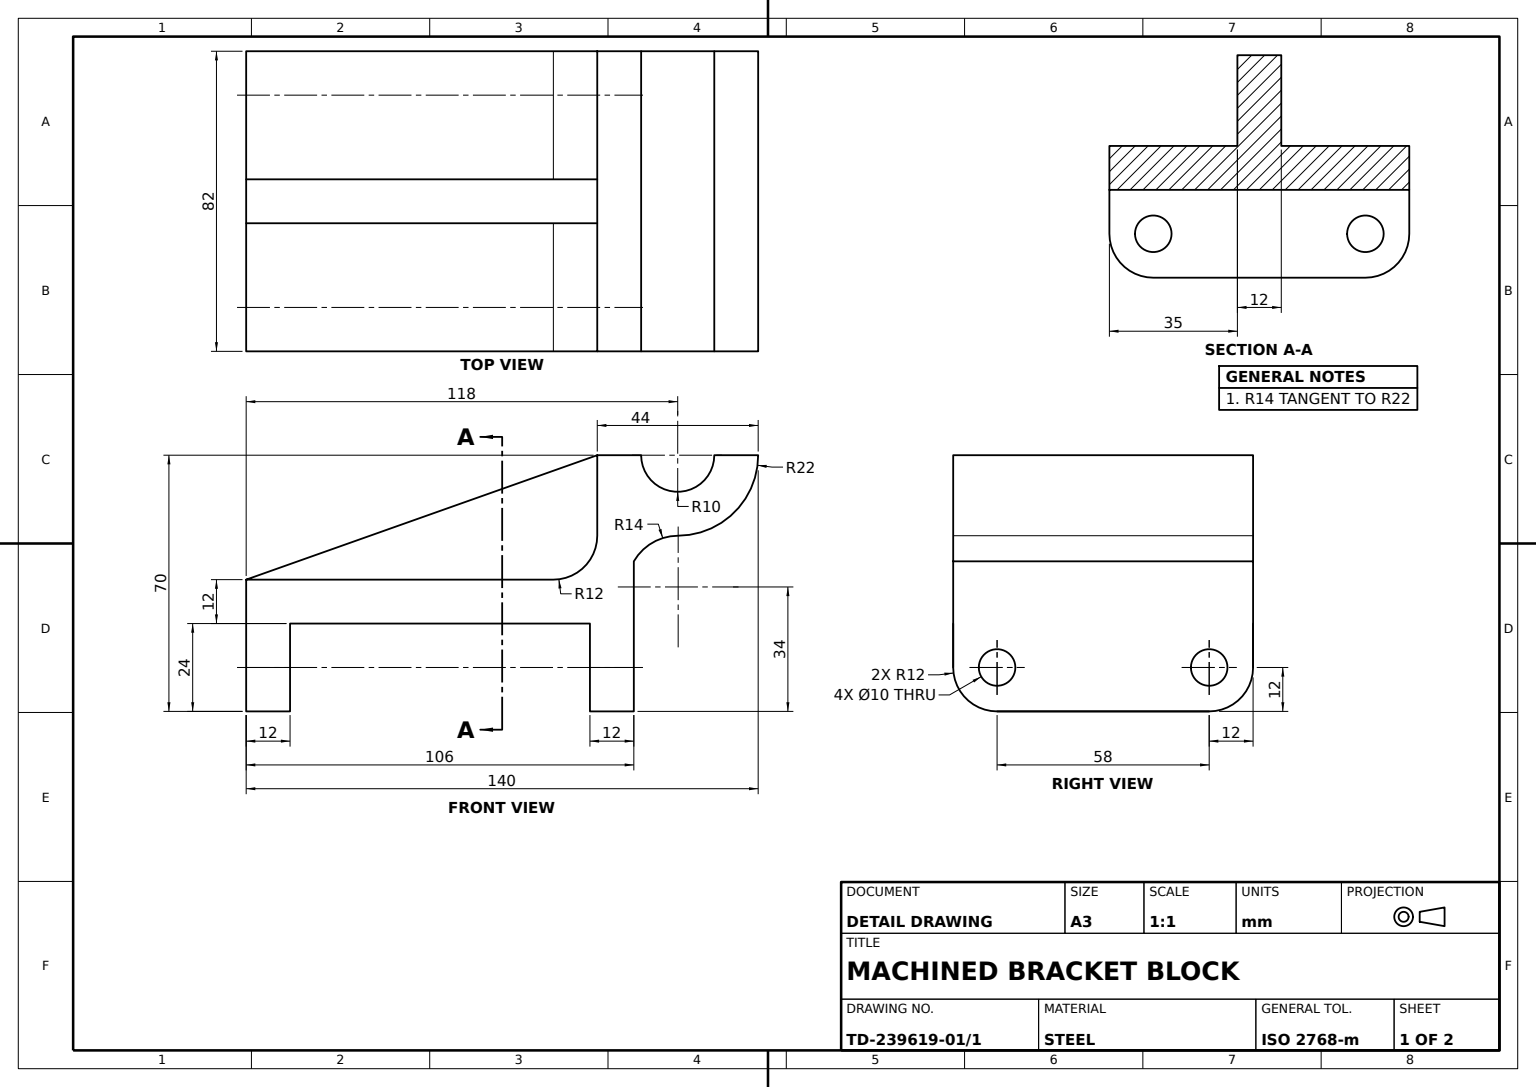
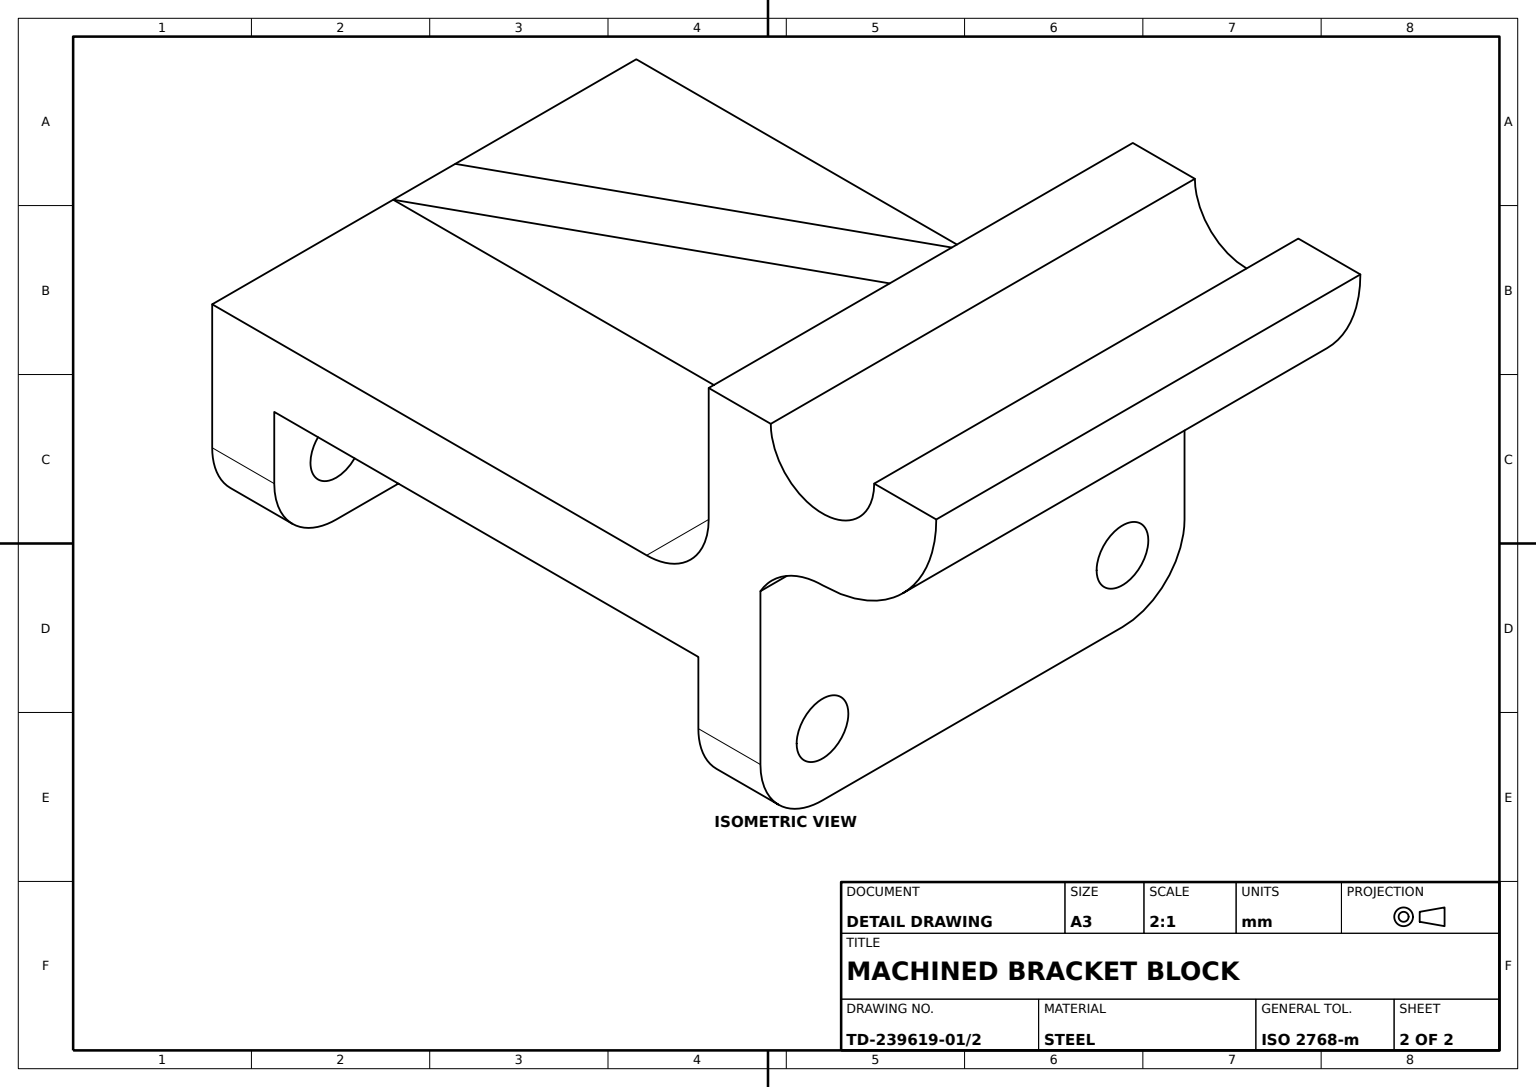
SolidWorks part; units mm, degrees
material "Plain Carbon Steel"
ref_plane "Front Plane" through (0, 0, 0) normal (0, 0, 1) x (1, 0, 0)
ref_plane "Top Plane" through (0, 0, 0) normal (0, 1, 0) x (1, 0, 0)
ref_plane "Right Plane" through (0, 0, 0) normal (1, 0, 0) x (0, 0, -1)
sketch "Base Plate Sketch" plane through (0, 0, 0) normal (0, 1, 0) x (1, 0, 0)
  line L1 (-53, -41) -> (53, -41)
  line L2 (-53, -41) -> (-53, 41)
  line L3 (-53, 41) -> (53, 41)
  line L4 (53, -41) -> (53, 41)
  line L5 (-53, -41) -> (53, 41) construction
  line L6 (-53, 41) -> (53, -41) construction
  point P0 (0, 0)
  dimension "D1" = 82
  dimension "D2" = 106
extrude "Base Plate" add sketch "Base Plate Sketch" along normal blind 12
sketch "Upright Wall Sketch" plane through (0, 0, 41) normal (0, 0, 1) x (1, 0, 0)
  line L1 (53, 12) -> (43, 12)
  line L2 (53, 12) -> (53, 46)
  line L3 (53, 46) -> (43, 46)
  line L4 (43, 12) -> (43, 46)
  dimension "D1" = 46
  dimension "D2" = 43
extrude "Upright Wall" add sketch "Upright Wall Sketch" against normal blind 82
fillet "Wall Root Fillet R12" radius 12 1 edges at (43, 12, 0)
sketch "Mounting Lug 1 Sketch" plane through (-53, 0, 0) normal (-1, 0, 0) x (0, 0, 1)
  line L1 (-41, 0) -> (41, 0)
  line L2 (-41, 0) -> (-41, -24)
  line L3 (-41, -24) -> (41, -24)
  line L4 (41, 0) -> (41, -24)
  dimension "D1" = 24
  dimension "D2" = 41
extrude "Mounting Lug 1" add sketch "Mounting Lug 1 Sketch" against normal blind 12
fillet "Lug 1 Corner Fillet R12" radius 12 2 edges at (-47, -24, -41) (-47, -24, 41)
sketch "Lug 1 Hole Sketch" plane through (-53, 0, 0) normal (-1, 0, 0) x (0, 0, 1)
  circle A0 centre (-29, -12) radius 5
  circle A1 centre (29, -12) radius 5
  dimension "D1" = 10
extrude "Lug 1 Mounting Hole" cut sketch "Lug 1 Hole Sketch" against normal through all
sketch "Mounting Lug 2 Sketch" plane through (53, 0, 0) normal (1, 0, 0) x (0, 0, -1)
  line L1 (-41, 0) -> (41, 0)
  line L2 (-41, 0) -> (-41, -24)
  line L3 (-41, -24) -> (41, -24)
  line L4 (41, 0) -> (41, -24)
  dimension "D1" = 82
  dimension "D2" = 24
extrude "Mounting Lug 2" add sketch "Mounting Lug 2 Sketch" against normal blind 12
fillet "Lug 2 Corner Fillet R12" radius 12 2 edges at (47, -24, -41) (47, -24, 41)
sketch "Lug 2 Hole Sketch" plane through (53, 0, 0) normal (1, 0, 0) x (0, 0, -1)
  circle A0 centre (-29, -12) radius 5
  circle A1 centre (29, -12) radius 5
  dimension "D1" = 10
  dimension "D2" = 10
extrude "Lug 2 Mounting Hole" cut sketch "Lug 2 Hole Sketch" against normal blind 12
ref_plane "Plane1" through (0, 0, 0) normal (0, 0, 1) x (1, 0, 0)
sketch "Side Support Sketch" plane through (0, 0, 0) normal (0, 0, 1) x (1, 0, 0)
  line L0 (-53, 12) -> (43, 46)
  line L1 (43, 46) -> (43, 24)
  line L2 (-53, 12) -> (31, 12)
  arc A0 (31, 12) -> (43, 24) centre (31, 24) ccw construction
  arc A1 (43, 24) -> (31, 12) centre (31, 24) cw
  dimension "D1" = 12
extrude "Side Support" add sketch "Side Support Sketch" along normal mid plane 12
sketch "Clamp Rail Profile Sketch" plane through (0, 0, 41) normal (0, 0, 1) x (1, 0, 0)
  line L0 (53, 46) -> (55, 46)
  line L1 (53, 46) -> (53, -12) construction
  line L2 (75, 46) -> (87, 46)
  line L3 (53, 46) -> (53, 17)
  arc A0 (55, 46) -> (75, 46) centre (65, 46) ccw
  arc A1 (65.0761, 24.0001) -> (87, 46) centre (65, 46) ccw
  arc A2 (53, 17) -> (65.0761, 24.0001) centre (65.1245, 10.0002) cw
  dimension "D1" = 20
  dimension "D3" = 44
  dimension "D4" = 14
  dimension "D2" = 12
  dimension "D5" = 12
  dimension "D6" = 44
extrude "Grooved Clamp Rail" add sketch "Clamp Rail Profile Sketch" against normal blind 82
